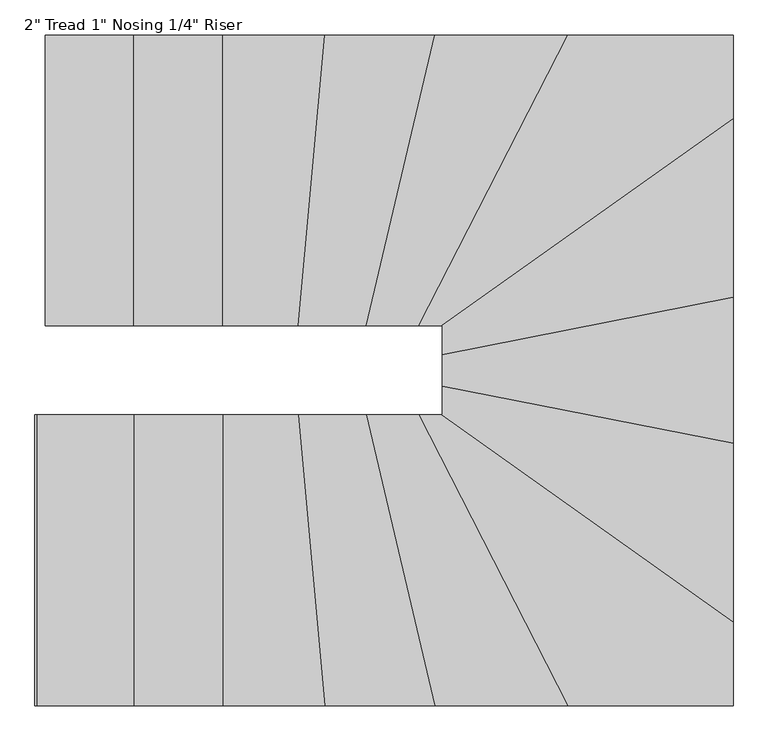
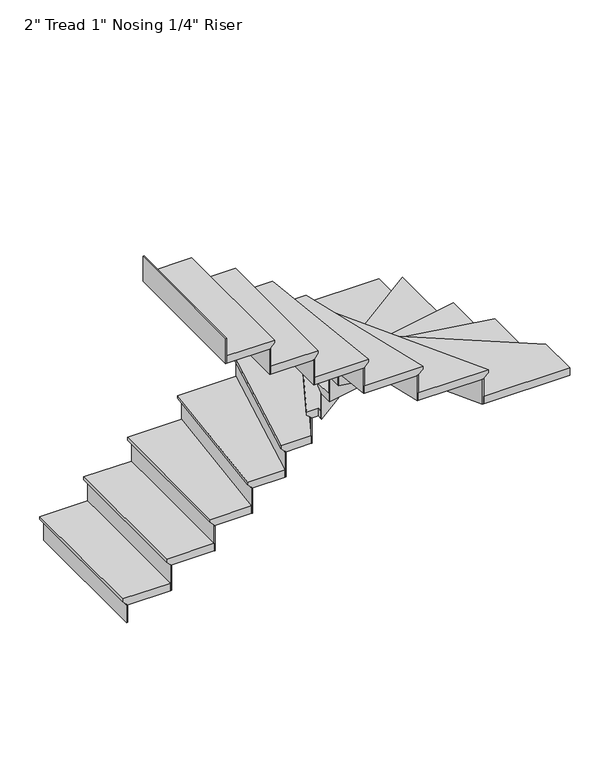
"""IFC4 building model written with IfcOpenShell, lengths in millimetres: stair flight geometry."""

from ifc_helpers import new_model, si_unit, origin, place, context, project, spatial, faceted_brep, source, transform, mapped, element, save


def stair_flight_f6c8c564(model_context):
    return source(origin(), model_context, "Body", "Brep", [
        faceted_brep([(-5447.3118598, 9571.7355643, 319.6166667), (-5447.3118598, 9571.7355643, 338.6666667), (-5447.3118598, 10486.1355643, 338.6666667), (-5447.3118598, 10486.1355643, 319.6166667), (-5421.9118598, 9571.7355643, 294.2166667), (-5421.9118598, 10486.1355643, 294.2166667), (-5142.5118598, 9571.7355643, 338.6666667), (-5142.5118598, 10486.1355643, 338.6666667), (-5421.9118598, 10486.1355643, 287.8666667), (-5142.5118598, 10486.1355643, 287.8666667), (-5142.5118598, 9571.7355643, 287.8666667), (-5421.9118598, 9571.7355643, 287.8666667)], [[[0, 1, 2, 3]], [[4, 0, 3, 5]], [[2, 1, 6, 7]], [[8, 9, 10, 11]], [[2, 7, 9, 8, 5, 3]], [[8, 11, 4, 5]], [[6, 1, 0, 4, 11, 10]], [[7, 6, 10, 9]]]),
        faceted_brep([(-5421.9118598, 9571.7355643, 287.8666667), (-5421.9118598, 9571.7355643, 169.3333333), (-5415.5618598, 9571.7355643, 169.3333333), (-5415.5618598, 9571.7355643, 287.8666667), (-5421.9118598, 10486.1355643, 287.8666667), (-5415.5618598, 10486.1355643, 287.8666667), (-5415.5618598, 10486.1355643, 169.3333333), (-5421.9118598, 10486.1355643, 169.3333333)], [[[0, 1, 2, 3]], [[4, 5, 6, 7]], [[1, 0, 4, 7]], [[2, 1, 7, 6]], [[3, 2, 6, 5]], [[0, 3, 5, 4]]]),
        faceted_brep([(-5142.5118598, 9571.7355643, 457.2), (-5142.5118598, 9571.7355643, 287.8666667), (-5136.1618598, 9571.7355643, 287.8666667), (-5136.1618598, 9571.7355643, 457.2), (-5142.5118598, 10486.1355643, 457.2), (-5136.1618598, 10486.1355643, 457.2), (-5136.1618598, 10486.1355643, 287.8666667), (-5142.5118598, 10486.1355643, 287.8666667)], [[[0, 1, 2, 3]], [[4, 5, 6, 7]], [[1, 0, 4, 7]], [[2, 1, 7, 6]], [[3, 2, 6, 5]], [[0, 3, 5, 4]]]),
        faceted_brep([(-5167.9118598, 10486.1355643, 508.0), (-5167.9118598, 9571.7355643, 508.0), (-4863.1118598, 9571.7355643, 508.0), (-4863.1118598, 10486.1355643, 508.0), (-5142.5118598, 10486.1355643, 457.2), (-4863.1118598, 10486.1355643, 457.2), (-4863.1118598, 9571.7355643, 457.2), (-5142.5118598, 9571.7355643, 457.2), (-5142.5118598, 10486.1355643, 463.55), (-5167.9118598, 10486.1355643, 488.95), (-5142.5118598, 9571.7355643, 463.55), (-5167.9118598, 9571.7355643, 488.95)], [[[0, 1, 2, 3]], [[4, 5, 6, 7]], [[0, 3, 5, 4, 8, 9]], [[4, 7, 10, 8]], [[2, 1, 11, 10, 7, 6]], [[3, 2, 6, 5]], [[11, 1, 0, 9]], [[10, 11, 9, 8]]]),
        faceted_brep([(-4863.1118598, 9571.7355643, 626.5333333), (-4863.1118598, 9571.7355643, 457.2), (-4856.7618598, 9571.7355643, 457.2), (-4856.7618598, 9571.7355643, 626.5333333), (-4863.1118598, 10486.1355643, 626.5333333), (-4856.7618598, 10486.1355643, 626.5333333), (-4856.7618598, 10486.1355643, 457.2), (-4863.1118598, 10486.1355643, 457.2)], [[[0, 1, 2, 3]], [[4, 5, 6, 7]], [[1, 0, 4, 7]], [[2, 1, 7, 6]], [[3, 2, 6, 5]], [[0, 3, 5, 4]]]),
        faceted_brep([(-4888.5118598, 10486.1355643, 677.3333333), (-4888.5118598, 9571.7355643, 677.3333333), (-4625.0854032, 9571.7355643, 677.3333333), (-4542.1296929, 10486.1355643, 677.3333333), (-4863.1118598, 10486.1355643, 626.5333333), (-4542.1296929, 10486.1355643, 626.5333333), (-4625.0854032, 9571.7355643, 626.5333333), (-4863.1118598, 9571.7355643, 626.5333333), (-4863.1118598, 10486.1355643, 632.8833333), (-4888.5118598, 10486.1355643, 658.2833333), (-4863.1118598, 9571.7355643, 632.8833333), (-4888.5118598, 9571.7355643, 658.2833333)], [[[0, 1, 2, 3]], [[4, 5, 6, 7]], [[0, 3, 5, 4, 8, 9]], [[4, 7, 10, 8]], [[2, 1, 11, 10, 7, 6]], [[3, 2, 6, 5]], [[11, 1, 0, 9]], [[10, 11, 9, 8]]]),
        faceted_brep([(-4625.0854032, 9571.7355643, 795.8666667), (-4625.0854032, 9571.7355643, 626.5333333), (-4618.7093253, 9571.7355643, 626.5333333), (-4618.7093253, 9571.7355643, 795.8666667), (-4542.1296929, 10486.1355643, 795.8666667), (-4535.753615, 10486.1355643, 795.8666667), (-4535.753615, 10486.1355643, 626.5333333), (-4542.1296929, 10486.1355643, 626.5333333)], [[[0, 1, 2, 3]], [[4, 5, 6, 7]], [[1, 0, 4, 7]], [[2, 1, 7, 6]], [[3, 2, 6, 5]], [[0, 3, 5, 4]]]),
        faceted_brep([(-4567.6340046, 10486.1355643, 846.6666667), (-4650.5897149, 9571.7355643, 846.6666667), (-4411.4822879, 9571.7355643, 846.6666667), (-4195.7467228, 10486.1355643, 846.6666667), (-4542.1296929, 10486.1355643, 795.8666667), (-4195.7467228, 10486.1355643, 795.8666667), (-4411.4822879, 9571.7355643, 795.8666667), (-4625.0854032, 9571.7355643, 795.8666667), (-4542.1296929, 10486.1355643, 802.2166667), (-4567.6340046, 10486.1355643, 827.6166667), (-4625.0854032, 9571.7355643, 802.2166667), (-4650.5897149, 9571.7355643, 827.6166667)], [[[0, 1, 2, 3]], [[4, 5, 6, 7]], [[0, 3, 5, 4, 8, 9]], [[4, 7, 10, 8]], [[2, 1, 11, 10, 7, 6]], [[3, 2, 6, 5]], [[11, 1, 0, 9]], [[10, 11, 9, 8]]]),
        faceted_brep([(-4411.4822879, 9571.7355643, 965.2), (-4411.4822879, 9571.7355643, 795.8666667), (-4404.9579493, 9571.7355643, 795.8666667), (-4404.9579493, 9571.7355643, 965.2), (-4195.7467228, 10486.1355643, 965.2), (-4189.2223842, 10486.1355643, 965.2), (-4189.2223842, 10486.1355643, 795.8666667), (-4195.7467228, 10486.1355643, 795.8666667)], [[[0, 1, 2, 3]], [[4, 5, 6, 7]], [[1, 0, 4, 7]], [[2, 1, 7, 6]], [[3, 2, 6, 5]], [[0, 3, 5, 4]]]),
        faceted_brep([(-4221.8440772, 10486.1355643, 1016.0), (-4437.5796423, 9571.7355643, 1016.0), (-4244.7041399, 9571.7355643, 1016.0), (-3775.8795186, 10486.1355643, 1016.0), (-4195.7467228, 10486.1355643, 965.2), (-3775.8795186, 10486.1355643, 965.2), (-4244.7041399, 9571.7355643, 965.2), (-4411.4822879, 9571.7355643, 965.2), (-4195.7467228, 10486.1355643, 971.55), (-4221.8440772, 10486.1355643, 996.95), (-4411.4822879, 9571.7355643, 971.55), (-4437.5796423, 9571.7355643, 996.95)], [[[0, 1, 2, 3]], [[4, 5, 6, 7]], [[0, 3, 5, 4, 8, 9]], [[4, 7, 10, 8]], [[2, 1, 11, 10, 7, 6]], [[3, 2, 6, 5]], [[11, 1, 0, 9]], [[10, 11, 9, 8]]]),
        faceted_brep([(-4244.7041399, 9571.7355643, 1134.5333333), (-4244.7041399, 9571.7355643, 965.2), (-4237.5681568, 9571.7355643, 965.2), (-4237.5681568, 9571.7355643, 1134.5333333), (-3775.8795186, 10486.1355643, 1134.5333333), (-3768.7435355, 10486.1355643, 1134.5333333), (-3768.7435355, 10486.1355643, 965.2), (-3775.8795186, 10486.1355643, 965.2)], [[[0, 1, 2, 3]], [[4, 5, 6, 7]], [[1, 0, 4, 7]], [[2, 1, 7, 6]], [[3, 2, 6, 5]], [[0, 3, 5, 4]]]),
        faceted_brep([(-3284.5801679, 10192.4544307, 1185.3333333), (-3284.5801679, 10486.1355643, 1185.3333333), (-3804.4234511, 10486.1355643, 1185.3333333), (-4273.2480725, 9571.7355643, 1185.3333333), (-4198.9801679, 9571.7355643, 1185.3333333), (-4198.9801679, 9542.1804815, 1185.3333333), (-3284.5801679, 10486.1355643, 1134.5333333), (-3284.5801679, 10192.4544307, 1134.5333333), (-4198.9801679, 9542.1804815, 1134.5333333), (-4198.9801679, 9571.7355643, 1134.5333333), (-4244.7041399, 9571.7355643, 1134.5333333), (-3775.8795186, 10486.1355643, 1134.5333333), (-4244.7041399, 9571.7355643, 1140.8833333), (-3775.8795186, 10486.1355643, 1140.8833333), (-4273.2480725, 9571.7355643, 1166.2833333), (-3804.4234511, 10486.1355643, 1166.2833333)], [[[0, 1, 2, 3, 4, 5]], [[6, 7, 8, 9, 10, 11]], [[1, 0, 7, 6]], [[11, 10, 12, 13]], [[4, 3, 14, 12, 10, 9]], [[0, 5, 8, 7]], [[14, 3, 2, 15]], [[12, 14, 15, 13]], [[2, 1, 6, 11, 13, 15]], [[5, 4, 9, 8]]]),
        faceted_brep([(-4198.9801679, 9542.1804815, 1303.8666667), (-4198.9801679, 9542.1804815, 1134.5333333), (-4198.9801679, 9534.3885067, 1134.5333333), (-4198.9801679, 9534.3885067, 1303.8666667), (-3284.5801679, 10192.4544307, 1303.8666667), (-3284.5801679, 10184.6624559, 1303.8666667), (-3284.5801679, 10184.6624559, 1134.5333333), (-3284.5801679, 10192.4544307, 1134.5333333)], [[[0, 1, 2, 3]], [[4, 5, 6, 7]], [[1, 0, 4, 7]], [[2, 1, 7, 6]], [[3, 2, 6, 5]], [[0, 3, 5, 4]]]),
        faceted_brep([(-3284.5801679, 10223.6223298, 1354.6666667), (-4198.9801679, 9573.3483807, 1354.6666667), (-4198.9801679, 9455.7263944, 1354.6666667), (-3284.5801679, 9635.9672508, 1354.6666667), (-3284.5801679, 10192.4544307, 1303.8666667), (-3284.5801679, 9635.9672508, 1303.8666667), (-4198.9801679, 9455.7263944, 1303.8666667), (-4198.9801679, 9542.1804815, 1303.8666667), (-3284.5801679, 10192.4544307, 1310.2166667), (-3284.5801679, 10223.6223298, 1335.6166667), (-4198.9801679, 9542.1804815, 1310.2166667), (-4198.9801679, 9573.3483807, 1335.6166667)], [[[0, 1, 2, 3]], [[4, 5, 6, 7]], [[0, 3, 5, 4, 8, 9]], [[4, 7, 10, 8]], [[2, 1, 11, 10, 7, 6]], [[3, 2, 6, 5]], [[11, 1, 0, 9]], [[10, 11, 9, 8]]]),
        faceted_brep([(-4198.9801679, 9455.7263944, 1473.2), (-4198.9801679, 9455.7263944, 1303.8666667), (-4198.9801679, 9449.254209, 1303.8666667), (-4198.9801679, 9449.254209, 1473.2), (-3284.5801679, 9635.9672508, 1473.2), (-3284.5801679, 9629.4950653, 1473.2), (-3284.5801679, 9629.4950653, 1303.8666667), (-3284.5801679, 9635.9672508, 1303.8666667)], [[[0, 1, 2, 3]], [[4, 5, 6, 7]], [[1, 0, 4, 7]], [[2, 1, 7, 6]], [[3, 2, 6, 5]], [[0, 3, 5, 4]]]),
        faceted_brep([(-3284.5801679, 9661.8559925, 1524.0), (-4198.9801679, 9481.6151362, 1524.0), (-4198.9801679, 9356.5672508, 1524.0), (-3284.5801679, 9176.3263944, 1524.0), (-3284.5801679, 9635.9672508, 1473.2), (-3284.5801679, 9176.3263944, 1473.2), (-4198.9801679, 9356.5672508, 1473.2), (-4198.9801679, 9455.7263944, 1473.2), (-3284.5801679, 9635.9672508, 1479.55), (-3284.5801679, 9661.8559925, 1504.95), (-4198.9801679, 9455.7263944, 1479.55), (-4198.9801679, 9481.6151362, 1504.95)], [[[0, 1, 2, 3]], [[4, 5, 6, 7]], [[0, 3, 5, 4, 8, 9]], [[4, 7, 10, 8]], [[3, 2, 6, 5]], [[11, 1, 0, 9]], [[10, 11, 9, 8]], [[2, 1, 11, 10, 7, 6]]]),
        faceted_brep([(-4198.9801679, 9356.5672508, 1642.5333333), (-4198.9801679, 9356.5672508, 1473.2), (-4198.9801679, 9350.0950653, 1473.2), (-4198.9801679, 9350.0950653, 1642.5333333), (-3284.5801679, 9176.3263944, 1642.5333333), (-3284.5801679, 9169.854209, 1642.5333333), (-3284.5801679, 9169.854209, 1473.2), (-3284.5801679, 9176.3263944, 1473.2)], [[[0, 1, 2, 3]], [[4, 5, 6, 7]], [[1, 0, 4, 7]], [[2, 1, 7, 6]], [[3, 2, 6, 5]], [[0, 3, 5, 4]]]),
        faceted_brep([(-3284.5801679, 9202.2151362, 1693.3333333), (-4198.9801679, 9382.4559925, 1693.3333333), (-4198.9801679, 9292.3355643, 1693.3333333), (-4245.0756424, 9292.3355643, 1693.3333333), (-3284.5801679, 8609.2808997, 1693.3333333), (-3284.5801679, 9176.3263944, 1642.5333333), (-3284.5801679, 8609.2808997, 1642.5333333), (-4245.0756424, 9292.3355643, 1642.5333333), (-4198.9801679, 9292.3355643, 1642.5333333), (-4198.9801679, 9356.5672508, 1642.5333333), (-3284.5801679, 9176.3263944, 1648.8833333), (-3284.5801679, 9202.2151362, 1674.2833333), (-4198.9801679, 9356.5672508, 1648.8833333), (-4198.9801679, 9382.4559925, 1674.2833333)], [[[0, 1, 2, 3, 4]], [[5, 6, 7, 8, 9]], [[0, 4, 6, 5, 10, 11]], [[5, 9, 12, 10]], [[2, 1, 13, 12, 9, 8]], [[4, 3, 7, 6]], [[13, 1, 0, 11]], [[12, 13, 11, 10]], [[3, 2, 8, 7]]]),
        faceted_brep([(-4245.0756424, 9292.3355643, 1811.8666667), (-4245.0756424, 9292.3355643, 1642.5333333), (-4256.0325349, 9292.3355643, 1642.5333333), (-4256.0325349, 9292.3355643, 1811.8666667), (-3284.5801679, 8609.2808997, 1811.8666667), (-3284.5801679, 8601.4889249, 1811.8666667), (-3284.5801679, 8601.4889249, 1642.5333333), (-3284.5801679, 8609.2808997, 1642.5333333)], [[[0, 1, 2, 3]], [[4, 5, 6, 7]], [[1, 0, 4, 7]], [[2, 1, 7, 6]], [[3, 2, 6, 5]], [[0, 3, 5, 4]]]),
        faceted_brep([(-3832.9673837, 8377.9355643, 1862.6666667), (-3284.5801679, 8377.9355643, 1862.6666667), (-3284.5801679, 8640.4487989, 1862.6666667), (-4201.2480725, 9292.3355643, 1862.6666667), (-4301.792005, 9292.3355643, 1862.6666667), (-3284.5801679, 8377.9355643, 1811.8666667), (-3832.9673837, 8377.9355643, 1811.8666667), (-4301.792005, 9292.3355643, 1811.8666667), (-4245.0756424, 9292.3355643, 1811.8666667), (-3284.5801679, 8609.2808997, 1811.8666667), (-4245.0756424, 9292.3355643, 1818.2166667), (-3284.5801679, 8609.2808997, 1818.2166667), (-4201.2480725, 9292.3355643, 1843.6166667), (-3284.5801679, 8640.4487989, 1843.6166667)], [[[0, 1, 2, 3, 4]], [[5, 6, 7, 8, 9]], [[1, 0, 6, 5]], [[9, 8, 10, 11]], [[4, 3, 12, 10, 8, 7]], [[0, 4, 7, 6]], [[12, 3, 2, 13]], [[10, 12, 13, 11]], [[2, 1, 5, 9, 11, 13]]]),
        faceted_brep([(-4301.792005, 9292.3355643, 1981.2), (-4301.792005, 9292.3355643, 1811.8666667), (-4308.9279881, 9292.3355643, 1811.8666667), (-4308.9279881, 9292.3355643, 1981.2), (-3832.9673837, 8377.9355643, 1981.2), (-3840.1033668, 8377.9355643, 1981.2), (-3840.1033668, 8377.9355643, 1811.8666667), (-3832.9673837, 8377.9355643, 1811.8666667)], [[[0, 1, 2, 3]], [[4, 5, 6, 7]], [[1, 0, 4, 7]], [[2, 1, 7, 6]], [[3, 2, 6, 5]], [[0, 3, 5, 4]]]),
        faceted_brep([(-3804.4234511, 8377.9355643, 2032.0), (-4273.2480725, 9292.3355643, 2032.0), (-4463.6769968, 9292.3355643, 2032.0), (-4247.9414317, 8377.9355643, 2032.0), (-3832.9673837, 8377.9355643, 1981.2), (-4247.9414317, 8377.9355643, 1981.2), (-4463.6769968, 9292.3355643, 1981.2), (-4301.792005, 9292.3355643, 1981.2), (-3832.9673837, 8377.9355643, 1987.55), (-3804.4234511, 8377.9355643, 2012.95), (-4301.792005, 9292.3355643, 1987.55), (-4273.2480725, 9292.3355643, 2012.95)], [[[0, 1, 2, 3]], [[4, 5, 6, 7]], [[0, 3, 5, 4, 8, 9]], [[4, 7, 10, 8]], [[2, 1, 11, 10, 7, 6]], [[3, 2, 6, 5]], [[11, 1, 0, 9]], [[10, 11, 9, 8]]]),
        faceted_brep([(-4463.6769968, 9292.3355643, 2150.5333333), (-4463.6769968, 9292.3355643, 1981.2), (-4470.2013354, 9292.3355643, 1981.2), (-4470.2013354, 9292.3355643, 2150.5333333), (-4247.9414317, 8377.9355643, 2150.5333333), (-4254.4657703, 8377.9355643, 2150.5333333), (-4254.4657703, 8377.9355643, 1981.2), (-4247.9414317, 8377.9355643, 1981.2)], [[[0, 1, 2, 3]], [[4, 5, 6, 7]], [[1, 0, 4, 7]], [[2, 1, 7, 6]], [[3, 2, 6, 5]], [[0, 3, 5, 4]]]),
        faceted_brep([(-4221.8440772, 8377.9355643, 2201.3333333), (-4437.5796423, 9292.3355643, 2201.3333333), (-4676.0940266, 9292.3355643, 2201.3333333), (-4593.1383163, 8377.9355643, 2201.3333333), (-4247.9414317, 8377.9355643, 2150.5333333), (-4593.1383163, 8377.9355643, 2150.5333333), (-4676.0940266, 9292.3355643, 2150.5333333), (-4463.6769968, 9292.3355643, 2150.5333333), (-4247.9414317, 8377.9355643, 2156.8833333), (-4221.8440772, 8377.9355643, 2182.2833333), (-4463.6769968, 9292.3355643, 2156.8833333), (-4437.5796423, 9292.3355643, 2182.2833333)], [[[0, 1, 2, 3]], [[4, 5, 6, 7]], [[0, 3, 5, 4, 8, 9]], [[4, 7, 10, 8]], [[2, 1, 11, 10, 7, 6]], [[3, 2, 6, 5]], [[11, 1, 0, 9]], [[10, 11, 9, 8]]]),
        faceted_brep([(-4676.0940266, 9292.3355643, 2319.8666667), (-4676.0940266, 9292.3355643, 2150.5333333), (-4682.4701045, 9292.3355643, 2150.5333333), (-4682.4701045, 9292.3355643, 2319.8666667), (-4593.1383163, 8377.9355643, 2319.8666667), (-4599.5143943, 8377.9355643, 2319.8666667), (-4599.5143943, 8377.9355643, 2150.5333333), (-4593.1383163, 8377.9355643, 2150.5333333)], [[[0, 1, 2, 3]], [[4, 5, 6, 7]], [[1, 0, 4, 7]], [[2, 1, 7, 6]], [[3, 2, 6, 5]], [[0, 3, 5, 4]]]),
        faceted_brep([(-4567.6340046, 8377.9355643, 2370.6666667), (-4650.5897149, 9292.3355643, 2370.6666667), (-4913.9118598, 9292.3355643, 2370.6666667), (-4913.9118598, 8377.9355643, 2370.6666667), (-4593.1383163, 8377.9355643, 2319.8666667), (-4913.9118598, 8377.9355643, 2319.8666667), (-4913.9118598, 9292.3355643, 2319.8666667), (-4676.0940266, 9292.3355643, 2319.8666667), (-4593.1383163, 8377.9355643, 2326.2166667), (-4567.6340046, 8377.9355643, 2351.6166667), (-4676.0940266, 9292.3355643, 2326.2166667), (-4650.5897149, 9292.3355643, 2351.6166667)], [[[0, 1, 2, 3]], [[4, 5, 6, 7]], [[0, 3, 5, 4, 8, 9]], [[4, 7, 10, 8]], [[2, 1, 11, 10, 7, 6]], [[3, 2, 6, 5]], [[11, 1, 0, 9]], [[10, 11, 9, 8]]]),
        faceted_brep([(-4913.9118598, 9292.3355643, 2489.2), (-4913.9118598, 9292.3355643, 2319.8666667), (-4920.2618598, 9292.3355643, 2319.8666667), (-4920.2618598, 9292.3355643, 2489.2), (-4913.9118598, 8377.9355643, 2489.2), (-4920.2618598, 8377.9355643, 2489.2), (-4920.2618598, 8377.9355643, 2319.8666667), (-4913.9118598, 8377.9355643, 2319.8666667)], [[[0, 1, 2, 3]], [[4, 5, 6, 7]], [[1, 0, 4, 7]], [[2, 1, 7, 6]], [[3, 2, 6, 5]], [[0, 3, 5, 4]]]),
        faceted_brep([(-4888.5118598, 8377.9355643, 2540.0), (-4888.5118598, 9292.3355643, 2540.0), (-5193.3118598, 9292.3355643, 2540.0), (-5193.3118598, 8377.9355643, 2540.0), (-4913.9118598, 8377.9355643, 2489.2), (-5193.3118598, 8377.9355643, 2489.2), (-5193.3118598, 9292.3355643, 2489.2), (-4913.9118598, 9292.3355643, 2489.2), (-4913.9118598, 8377.9355643, 2495.55), (-4888.5118598, 8377.9355643, 2520.95), (-4913.9118598, 9292.3355643, 2495.55), (-4888.5118598, 9292.3355643, 2520.95)], [[[0, 1, 2, 3]], [[4, 5, 6, 7]], [[0, 3, 5, 4, 8, 9]], [[4, 7, 10, 8]], [[2, 1, 11, 10, 7, 6]], [[3, 2, 6, 5]], [[11, 1, 0, 9]], [[10, 11, 9, 8]]]),
        faceted_brep([(-5193.3118598, 9292.3355643, 2658.5333333), (-5193.3118598, 9292.3355643, 2489.2), (-5199.6618598, 9292.3355643, 2489.2), (-5199.6618598, 9292.3355643, 2658.5333333), (-5193.3118598, 8377.9355643, 2658.5333333), (-5199.6618598, 8377.9355643, 2658.5333333), (-5199.6618598, 8377.9355643, 2489.2), (-5193.3118598, 8377.9355643, 2489.2)], [[[0, 1, 2, 3]], [[4, 5, 6, 7]], [[1, 0, 4, 7]], [[2, 1, 7, 6]], [[3, 2, 6, 5]], [[0, 3, 5, 4]]]),
        faceted_brep([(-5472.7118598, 9292.3355643, 2827.8666667), (-5472.7118598, 9292.3355643, 2658.5333333), (-5479.0618598, 9292.3355643, 2658.5333333), (-5479.0618598, 9292.3355643, 2827.8666667), (-5472.7118598, 8377.9355643, 2827.8666667), (-5479.0618598, 8377.9355643, 2827.8666667), (-5479.0618598, 8377.9355643, 2658.5333333), (-5472.7118598, 8377.9355643, 2658.5333333)], [[[0, 1, 2, 3]], [[4, 5, 6, 7]], [[1, 0, 4, 7]], [[2, 1, 7, 6]], [[3, 2, 6, 5]], [[0, 3, 5, 4]]]),
        faceted_brep([(-5167.9118598, 8377.9355643, 2709.3333333), (-5167.9118598, 9292.3355643, 2709.3333333), (-5472.7118598, 9292.3355643, 2709.3333333), (-5472.7118598, 8377.9355643, 2709.3333333), (-5193.3118598, 8377.9355643, 2658.5333333), (-5472.7118598, 8377.9355643, 2658.5333333), (-5472.7118598, 9292.3355643, 2658.5333333), (-5193.3118598, 9292.3355643, 2658.5333333), (-5193.3118598, 8377.9355643, 2664.8833333), (-5167.9118598, 8377.9355643, 2690.2833333), (-5193.3118598, 9292.3355643, 2664.8833333), (-5167.9118598, 9292.3355643, 2690.2833333)], [[[0, 1, 2, 3]], [[4, 5, 6, 7]], [[0, 3, 5, 4, 8, 9]], [[4, 7, 10, 8]], [[2, 1, 11, 10, 7, 6]], [[3, 2, 6, 5]], [[11, 1, 0, 9]], [[10, 11, 9, 8]]]),
    ])


if __name__ == "__main__":
    model = new_model("IFC4")
    model_context = context("Model", 3, world=origin())
    ifc_project = project(units=[si_unit("LENGTHUNIT", "METRE", prefix="MILLI")], contexts=[model_context])
    site = spatial("IfcSite", under=ifc_project)
    building = spatial("IfcBuilding", under=site)
    placement = place(None, origin())
    stair_flight_shape = stair_flight_f6c8c564(model_context)
    element("IfcStairFlight", 1, ObjectType="2\" Tread 1\" Nosing 1/4\" Riser", at=placement, inside=building, context=model_context, shape_type="MappedRepresentation", body=[
        mapped(stair_flight_shape, transform((0.0, 0.0, 0.0), x_axis=(1.0, 0.0, 0.0), y_axis=(0.0, 1.0, 0.0), z_axis=(0.0, 0.0, 1.0))),
    ])
    save(model, "model.ifc")
